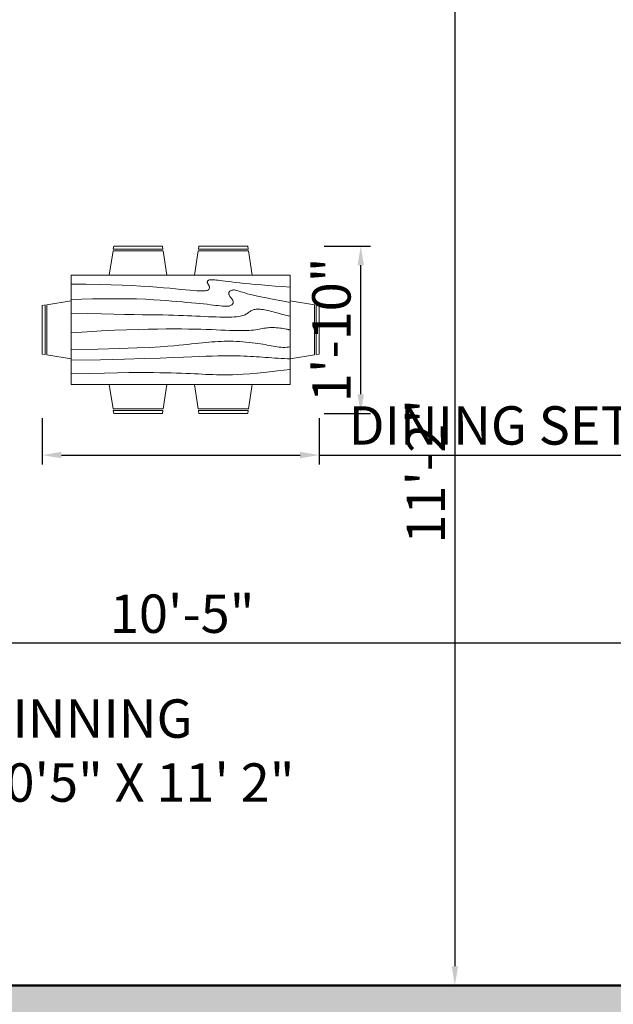
# Model space of a CAD drawing. Units: millimetres. Extents: x 2784 to 3697, y 603 to 1406.
# Tile 5 of 10: x 3013 to 3091, y 1077 to 1205. Entities that reach past the tile are written whole.
import ezdxf

# ---------------------------------------------------------------- set-up
doc = ezdxf.new("R2010")
doc.units = ezdxf.units.MM
for name, color, linetype, lineweight in [('A-ANNO-DIMS', 140, 'Continuous', 18), ('A-AREA-IDEN', 150, 'Continuous', 25), ('A-FURN', 80, 'Continuous', 18), ('A-WALL', 2, 'Continuous', 50), ('A-WALL-PATT', 8, 'Continuous', 13)]:
    doc.layers.add(name, color=color, linetype=linetype, lineweight=lineweight)
doc.styles.get("Standard").update_dxf_attribs({"font": 'arial.ttf'})
doc.dimstyles.new('ISO-25', dxfattribs={"dimtxt": 5, "dimasz": 2.5, "dimexe": 1.25, "dimexo": 0.625, "dimtad": 1, "dimdec": 0, "dimlunit": 3, "dimtxsty": 'Standard', "dimcen": 2.5, "dimadec": 0, "dimazin": 0, "dimtfac": 1, "dimtdec": 0, "dimtmove": 0, "dimatfit": 3, "dimfxl": 1, "dimarcsym": 0})

# ---------------------------------------------------------------- blocks, each defined once
blk = doc.blocks.new('Dining Set - 36 x 72 in.')
for p, q in [((-22.2343, 26.00059), (-23.4847, 17.99762)), ((-22.2304, 26), (-5.7608, 26)), ((-22, 27.5), (-22.1562, 26.50042)), ((-5.8416, 26.5), (-22.1534, 26.5)), ((-22, 27.5), (-6, 27.5)), ((-5.8437, 26.49966), (-6, 27.5)), ((-4.5152, 17.99762), (-5.7655, 25.99926)), ((5.7657, 26.00059), (4.5153, 17.99762)), ((5.7696, 26), (22.2392, 26)), ((6, 27.5), (5.8438, 26.50042)), ((22.1584, 26.5), (5.8466, 26.5)), ((6, 27.5), (22, 27.5)), ((22.1563, 26.49966), (22, 27.5)), ((23.4848, 17.99762), (22.2345, 25.99926)), ((36, 18), (-36, 18)), ((-36, 18), (-36, -18)), ((36, -18), (36, 18)), ((-45.5, 8), (-44.5004, 8.15617)), ((-45.5, 8), (-45.5, -8)), ((-44.5, -8.15843), (-44.5, 8.15338)), ((-44.0006, 8.23428), (-35.9976, 9.48474)), ((-44, 8.23041), (-44, -8.23915)), ((44.0006, 8.23428), (35.9976, 9.48474)), ((44, 8.23041), (44, -8.23915)), ((44.5, -8.15843), (44.5, 8.15338)), ((45.5, 8), (44.5005, 8.15617)), ((45.5, 8), (45.5, -8)), ((-44.4997, -8.15631), (-45.5, -8)), ((-35.9976, -9.48476), (-43.9993, -8.2345)), ((35.9976, -9.48476), (43.9993, -8.2345)), ((44.4997, -8.15631), (45.5, -8)), ((-36, -18), (36, -18)), ((-22.2343, -26.0006), (-23.4847, -17.99762)), ((-4.5152, -17.99762), (-5.7655, -25.99928)), ((5.7657, -26.0006), (4.5153, -17.99762)), ((23.4848, -17.99762), (22.2345, -25.99928)), ((-22.2304, -26), (-5.7608, -26)), ((-22, -27.5), (-22.1562, -26.50044)), ((-5.8416, -26.5), (-22.1534, -26.5)), ((-22, -27.5), (-6, -27.5)), ((-5.8437, -26.49967), (-6, -27.5)), ((5.7696, -26), (22.2392, -26)), ((6, -27.5), (5.8438, -26.50044)), ((22.1584, -26.5), (5.8466, -26.5)), ((6, -27.5), (22, -27.5)), ((22.1563, -26.49967), (22, -27.5))]:
    blk.add_line(p, q)
for points in [[(-36, 15), (-31.1772, 14.97754), (-26.8079, 14.91406), (-22.8538, 14.81543), (-19.276, 14.6875), (-16.0362, 14.53613), (-13.0957, 14.36718), (-10.4159, 14.18652), (-7.9583, 14), (-5.6904, 13.81315), (-3.6035, 13.63021), (-1.6954, 13.45508), (0.0365, 13.29166), (1.5945, 13.14388), (2.9811, 13.01562), (4.1988, 12.9108), (5.25, 12.83333), (6.1393, 12.78613), (6.8802, 12.76823), (7.4883, 12.77767), (7.9792, 12.8125), (8.3685, 12.87077), (8.6719, 12.95052), (8.9049, 13.0498), (9.0833, 13.16666), (9.2205, 13.29899), (9.3216, 13.44401), (9.3895, 13.59879), (9.4271, 13.76041), (9.4373, 13.92594), (9.4232, 14.09245), (9.3875, 14.257), (9.3333, 14.41666), (9.2638, 14.56917), (9.1836, 14.71484), (9.0975, 14.85465), (9.0104, 14.98958), (8.9272, 15.1206), (8.8529, 15.2487), (8.7922, 15.37483), (8.75, 15.5), (8.7305, 15.62467), (8.7344, 15.74739), (8.7617, 15.86621), (8.8125, 15.97916), (8.8867, 16.08431), (8.9844, 16.17968), (9.1055, 16.26334), (9.25, 16.33333), (9.4189, 16.38802), (9.6172, 16.42708), (9.8506, 16.45052), (10.125, 16.45833), (10.4463, 16.45052), (10.8203, 16.42708), (11.2529, 16.38802), (11.75, 16.33333), (12.3184, 16.26318), (12.9694, 16.17838), (13.7151, 16.07991), (14.5677, 15.96875), (15.5395, 15.84586), (16.6426, 15.71224), (17.8893, 15.56884), (19.2917, 15.41666), (20.859, 15.25667), (22.5879, 15.08984), (24.4721, 14.91715), (26.5052, 14.73958), (28.6809, 14.5581), (30.9929, 14.3737), (33.4347, 14.18733), (36, 14)], [(-36, 10), (-28.9766, 10.14274), (-23.1725, 10.20442), (-18.4241, 10.19775), (-14.5677, 10.13541), (-11.4399, 10.03011), (-8.877, 9.89453), (-6.7154, 9.74137), (-4.7917, 9.58333), (-2.9698, 9.43082), (-1.2246, 9.28515), (0.4415, 9.14534), (2.026, 9.01041), (3.5266, 8.87939), (4.9408, 8.7513), (6.266, 8.62516), (7.5, 8.5), (8.6411, 8.37549), (9.6914, 8.2539), (10.6538, 8.13818), (11.5312, 8.03125), (12.3267, 7.93603), (13.043, 7.85547), (13.6831, 7.79248), (14.25, 7.75), (14.7471, 7.7303), (15.1797, 7.73307), (15.5537, 7.75732), (15.875, 7.80208), (16.1494, 7.86637), (16.3828, 7.94922), (16.5811, 8.04964), (16.75, 8.16666), (16.8944, 8.29915), (17.0143, 8.44531), (17.1089, 8.60319), (17.1771, 8.77083), (17.218, 8.94629), (17.2305, 9.1276), (17.2137, 9.31282), (17.1667, 9.5), (17.0895, 9.6875), (16.987, 9.875), (16.8649, 10.0625), (16.7292, 10.25), (16.5856, 10.4375), (16.4401, 10.625), (16.2985, 10.8125), (16.1667, 11), (16.05, 11.18733), (15.9518, 11.3737), (15.8752, 11.5581), (15.8229, 11.73958), (15.798, 11.91715), (15.8034, 12.08984), (15.842, 12.25667), (15.9167, 12.41666), (16.0295, 12.56836), (16.1784, 12.70833), (16.3605, 12.83268), (16.5729, 12.9375), (16.8127, 13.01888), (17.0768, 13.07291), (17.3625, 13.0957), (17.6667, 13.08333), (17.9894, 13.03312), (18.3418, 12.94726), (18.7382, 12.82918), (19.1927, 12.68229), (19.7195, 12.51001), (20.3327, 12.31575), (21.0465, 12.10294), (21.875, 11.875), (22.8357, 11.63354), (23.959, 11.37304), (25.2786, 11.08618), (26.8282, 10.76562), (28.6414, 10.40405), (30.752, 9.99414), (33.1936, 9.52856), (36, 9)], [(-36, 5.5), (-30.7157, 5.3348), (-26.069, 5.20963), (-21.9946, 5.11767), (-18.4271, 5.05208), (-15.3009, 5.00602), (-12.5508, 4.97265), (-10.1112, 4.94515), (-7.9167, 4.91666), (-5.909, 4.88167), (-4.0586, 4.83984), (-2.3429, 4.79215), (-0.7396, 4.73958), (0.7739, 4.6831), (2.22, 4.6237), (3.6213, 4.56233), (5, 4.5), (6.373, 4.43782), (7.7344, 4.3776), (9.0723, 4.32129), (10.375, 4.27083), (11.6309, 4.22819), (12.8281, 4.19531), (13.9551, 4.17415), (15, 4.16666), (15.954, 4.17448), (16.819, 4.19791), (17.6001, 4.23698), (18.3021, 4.29166), (18.9299, 4.36198), (19.4883, 4.44791), (19.9823, 4.54948), (20.4167, 4.66666), (20.7969, 4.79899), (21.1302, 4.94401), (21.4245, 5.09879), (21.6875, 5.26041), (21.9271, 5.42594), (22.1511, 5.59245), (22.3672, 5.757), (22.5834, 5.91666), (22.8065, 6.06868), (23.0404, 6.21093), (23.2879, 6.34147), (23.5521, 6.45833), (23.8358, 6.55957), (24.142, 6.64323), (24.4735, 6.70735), (24.8334, 6.75), (25.2235, 6.76969), (25.642, 6.76692), (26.0858, 6.74267), (26.5521, 6.69791), (27.0379, 6.63362), (27.5404, 6.55078), (28.0565, 6.45036), (28.5834, 6.33333), (29.1242, 6.19987), (29.7071, 6.04687), (30.3661, 5.87044), (31.1354, 5.66666), (32.0493, 5.43164), (33.142, 5.16146), (34.4475, 4.85221), (36, 4.5)], [(-36, -1), (-30.7915, -0.6591), (-26.0195, -0.38216), (-21.6519, -0.16284), (-17.6563, 0.00521), (-14.0005, 0.12833), (-10.6523, 0.21289), (-7.5796, 0.26522), (-4.75, 0.29166), (-2.134, 0.29793), (0.2878, 0.28711), (2.5317, 0.26163), (4.6146, 0.22396), (6.5529, 0.17651), (8.3633, 0.12174), (10.0623, 0.06209), (11.6667, 0), (13.1899, -0.06201), (14.6341, -0.1211), (15.9982, -0.17432), (17.2813, -0.21875), (18.4823, -0.25147), (19.6003, -0.26953), (20.6343, -0.27002), (21.5834, -0.25), (22.4481, -0.20768), (23.2357, -0.14584), (23.9549, -0.06836), (24.6146, 0.02083), (25.2235, 0.11784), (25.7904, 0.21875), (26.3241, 0.31966), (26.8334, 0.41666), (27.3265, 0.50618), (27.8099, 0.58593), (28.2894, 0.65397), (28.7709, 0.70833), (29.2601, 0.74707), (29.763, 0.76823), (30.2855, 0.76985), (30.8334, 0.75), (31.4088, 0.70784), (31.9994, 0.64713), (32.589, 0.57275), (33.1615, 0.48958), (33.7008, 0.4025), (34.1908, 0.3164), (34.6153, 0.23616), (34.9584, 0.16666), (35.2099, 0.11165), (35.3848, 0.07031), (35.504, 0.04069), (35.5886, 0.02083), (35.6594, 0.00879), (35.7377, 0.0026), (35.8442, 0.00032), (36, 0)], [(-36, -6.5), (-27.1843, -6.31267), (-20.084, -6.1263), (-14.469, -5.9419), (-10.1094, -5.76042), (-6.7752, -5.58285), (-4.2363, -5.41016), (-2.2629, -5.24333), (-0.625, -5.08334), (0.8708, -4.93099), (2.2715, -4.78646), (3.5872, -4.64974), (4.8281, -4.52084), (6.0046, -4.39974), (7.127, -4.28646), (8.2053, -4.18099), (9.25, -4.08334), (10.2705, -3.99382), (11.2734, -3.91407), (12.2647, -3.84603), (13.25, -3.79167), (14.2354, -3.75293), (15.2266, -3.73177), (16.2295, -3.73015), (17.25, -3.75), (18.2912, -3.79248), (19.3451, -3.85547), (20.4009, -3.93604), (21.4479, -4.03125), (22.4754, -4.13819), (23.4727, -4.25391), (24.4289, -4.37549), (25.3334, -4.5), (26.1785, -4.62492), (26.9694, -4.74935), (27.7145, -4.87281), (28.4219, -4.99479), (29.1, -5.11483), (29.7572, -5.23242), (30.4016, -5.34709), (31.0417, -5.45834), (31.6837, -5.56437), (32.3262, -5.65821), (32.9658, -5.73153), (33.599, -5.77604), (34.2224, -5.78345), (34.8327, -5.74545), (35.4264, -5.65373), (36, -5.5)], [(-36, -10), (-26.4022, -9.81299), (-18.4675, -9.62891), (-11.9839, -9.45069), (-6.7396, -9.28125), (-2.5226, -9.12354), (0.8789, -8.98047), (3.6769, -8.85498), (6.0833, -8.75), (8.2767, -8.66765), (10.3021, -8.60677), (12.1712, -8.56543), (13.8958, -8.54167), (15.4876, -8.53353), (16.9583, -8.53907), (18.3197, -8.55632), (19.5834, -8.58334), (20.7616, -8.61841), (21.8685, -8.66081), (22.9188, -8.71004), (23.9271, -8.76563), (24.9081, -8.82707), (25.8763, -8.89388), (26.8465, -8.96558), (27.8334, -9.04167), (28.8474, -9.12118), (29.8828, -9.20117), (30.93, -9.27824), (31.9792, -9.34896), (33.0205, -9.40991), (34.0443, -9.45768), (35.0407, -9.48885), (36, -9.5)], [(-36, -14.5), (-30.0881, -14.33513), (-25.0332, -14.21224), (-20.7312, -14.12647), (-17.0781, -14.07292), (-13.97, -14.04671), (-11.3027, -14.04297), (-8.9724, -14.05681), (-6.875, -14.08334), (-4.9224, -14.11833), (-3.0905, -14.16016), (-1.3709, -14.20785), (0.2448, -14.26042), (1.7647, -14.3169), (3.1973, -14.3763), (4.5507, -14.43767), (5.8333, -14.5), (7.0554, -14.5621), (8.235, -14.62175), (9.3922, -14.67652), (10.5469, -14.72396), (11.7192, -14.76164), (12.929, -14.78711), (14.1965, -14.79794), (15.5417, -14.79167), (16.9933, -14.76424), (18.6152, -14.70508), (20.4804, -14.60197), (22.6615, -14.44271), (25.2312, -14.21509), (28.2624, -13.9069), (31.8277, -13.50594), (36, -13)]]:
    blk.add_lwpolyline(points)
blk = doc.blocks.new('*D36')
at = {"layer": 'A-ANNO-DIMS', "color": 0, "lineweight": -2, "transparency": 16777216}
for p, q in [((2971.91, 1166.33), (2971.91, 1122.59)), ((3096.91, 1166.33), (3096.91, 1122.59)), ((3094.41, 1123.84), (2974.41, 1123.84))]:
    blk.add_line(p, q, dxfattribs=at)
at = {"layer": 'A-ANNO-DIMS', "color": 0, "transparency": 16777216}
for points in [[(2974.41, 1124.26), (2974.41, 1123.43), (2971.91, 1123.84)], [(3094.41, 1124.26), (3094.41, 1123.43), (3096.91, 1123.84)]]:
    blk.add_solid(points, dxfattribs=at)
at = {"layer": 'Defpoints', "color": 0, "transparency": 16777216}
for p in [(2971.91, 1166.96), (3096.91, 1166.96), (2971.91, 1123.84)]:
    blk.add_point(p, dxfattribs=at)
at = {"layer": 'A-ANNO-DIMS', "color": 0, "transparency": 16777216, "insert": (3034.41, 1127.02), "char_height": 5, "attachment_point": 5}
blk.add_mtext('10\'-5"', dxfattribs=at)
blk = doc.blocks.new('*D37')
at = {"layer": 'A-ANNO-DIMS', "color": 0, "lineweight": -2, "transparency": 16777216}
for p, q in [((3069.6, 1213.23), (3068.7, 1213.23)), ((3069.95, 1210.73), (3069.95, 1081.73)), ((3069.6, 1079.23), (3068.7, 1079.23))]:
    blk.add_line(p, q, dxfattribs=at)
at = {"layer": 'A-ANNO-DIMS', "color": 0, "transparency": 16777216}
for points in [[(3069.53, 1210.73), (3070.37, 1210.73), (3069.95, 1213.23)], [(3069.53, 1081.73), (3070.37, 1081.73), (3069.95, 1079.23)]]:
    blk.add_solid(points, dxfattribs=at)
at = {"layer": 'Defpoints', "color": 0, "transparency": 16777216}
for p in [(3070.22, 1213.23), (3069.95, 1079.23), (3070.22, 1079.23)]:
    blk.add_point(p, dxfattribs=at)
at = {"layer": 'A-ANNO-DIMS', "color": 0, "transparency": 16777216, "insert": (3066.81, 1146.23), "char_height": 5, "attachment_point": 5, "rotation": 90}
blk.add_mtext('11\'-2"', dxfattribs=at)
blk = doc.blocks.new('*D74')
at = {"layer": 'A-ANNO-DIMS', "color": 0, "lineweight": -2, "transparency": 16777216}
for p, q in [((3016.17, 1153.13), (3016.17, 1147.09)), ((3052.27, 1153.13), (3052.27, 1147.09)), ((3018.67, 1148.34), (3049.77, 1148.34)), ((3052.27, 1148.34), (3110.98, 1148.34))]:
    blk.add_line(p, q, dxfattribs=at)
at = {"layer": 'A-ANNO-DIMS', "color": 0, "transparency": 16777216}
for points in [[(3018.67, 1148.76), (3018.67, 1147.92), (3016.17, 1148.34)], [(3049.77, 1148.76), (3049.77, 1147.92), (3052.27, 1148.34)]]:
    blk.add_solid(points, dxfattribs=at)
at = {"layer": 'Defpoints', "color": 0, "transparency": 16777216}
for p in [(3016.17, 1153.76), (3052.27, 1153.76), (3052.27, 1148.34)]:
    blk.add_point(p, dxfattribs=at)
at = {"layer": 'A-ANNO-DIMS', "color": 0, "transparency": 16777216, "insert": (3082.87, 1151.55), "char_height": 5, "attachment_point": 5}
blk.add_mtext('DINING SET 3\'-0"', dxfattribs=at)
blk = doc.blocks.new('*D75')
at = {"layer": 'A-ANNO-DIMS', "color": 0, "lineweight": -2, "transparency": 16777216}
for p, q in [((3052.9, 1175.57), (3058.94, 1175.57)), ((3057.69, 1156.26), (3057.69, 1173.07)), ((3052.9, 1153.76), (3058.94, 1153.76))]:
    blk.add_line(p, q, dxfattribs=at)
at = {"layer": 'A-ANNO-DIMS', "color": 0, "transparency": 16777216}
for points in [[(3057.27, 1173.07), (3058.1, 1173.07), (3057.69, 1175.57)], [(3057.27, 1156.26), (3058.1, 1156.26), (3057.69, 1153.76)]]:
    blk.add_solid(points, dxfattribs=at)
at = {"layer": 'Defpoints', "color": 0, "transparency": 16777216}
for p in [(3052.27, 1175.57), (3057.69, 1175.57), (3052.27, 1153.76)]:
    blk.add_point(p, dxfattribs=at)
at = {"layer": 'A-ANNO-DIMS', "color": 0, "transparency": 16777216, "insert": (3054.51, 1164.66), "char_height": 5, "attachment_point": 5, "rotation": 90}
blk.add_mtext('1\'-10"', dxfattribs=at)

msp = doc.modelspace()

# ---------------------------------------------------------------- hatches: boundary and pattern name
at = {"layer": 'A-WALL-PATT'}
h = msp.add_hatch(color=256, dxfattribs=at)
h.dxf.hatch_style = 1
h.paths.add_polyline_path([(2869.53, 1356.23), (2839.91, 1356.23), (2839.91, 1347.23), (2869.53, 1347.23)])
h.paths.add_polyline_path([(2839.91, 1356.23), (2830.91, 1356.23), (2830.91, 1347.23), (2839.91, 1347.23)])
h.paths.add_polyline_path([(2839.91, 1347.23), (2830.91, 1347.23), (2830.91, 1314.23), (2839.91, 1314.23)])
h.paths.add_polyline_path([(2839.91, 1268.19), (2830.91, 1268.19), (2830.91, 1222.23), (2839.91, 1222.23)])
h.paths.add_polyline_path([(2839.91, 1222.23), (2830.91, 1222.23), (2830.91, 1213.23), (2839.91, 1213.23)])
h.paths.add_polyline_path([(2962.91, 1222.23), (2839.91, 1222.23), (2839.91, 1213.23), (2962.91, 1213.23)])
h.paths.add_polyline_path([(2971.91, 1222.23), (2962.91, 1222.23), (2962.91, 1213.23), (2971.91, 1213.23)])
h.paths.add_polyline_path([(2971.91, 1263.23), (2962.91, 1263.23), (2962.91, 1254.23), (2971.91, 1254.23)])
h.paths.add_polyline_path([(2971.91, 1347.23), (2962.91, 1347.23), (2962.91, 1263.23), (2971.91, 1263.23)])
h.paths.add_polyline_path([(2971.91, 1356.23), (2962.91, 1356.23), (2962.91, 1347.23), (2971.91, 1347.23)])
h.paths.add_polyline_path([(2962.91, 1356.23), (2913.7, 1356.23), (2913.7, 1347.23), (2962.91, 1347.23)])
h.paths.add_polyline_path([(2982.62, 1356.23), (2971.91, 1356.23), (2971.91, 1347.23), (2982.62, 1347.23)])
h.paths.add_polyline_path([(3019.91, 1356.23), (3004.44, 1356.23), (3004.44, 1347.23), (3019.91, 1347.23)])
h.paths.add_polyline_path([(3028.91, 1356.23), (3019.91, 1356.23), (3019.91, 1347.23), (3028.91, 1347.23)])
h.paths.add_polyline_path([(3028.91, 1347.23), (3019.91, 1347.23), (3019.91, 1287.35, -0.06506), (3026.12, 1288.16), (3028.91, 1288.16)])
h.paths.add_polyline_path([(3019.91, 1263.23), (2971.91, 1263.23), (2971.91, 1254.23), (3019.91, 1254.23)])
h.paths.add_polyline_path([(3028.91, 1263.23), (3019.91, 1263.23), (3019.91, 1254.23), (3028.91, 1254.23)])
h.paths.add_polyline_path([(3028.91, 1254.23), (3019.91, 1254.23), (3019.91, 1222.23), (3028.91, 1222.23)])
h.paths.add_polyline_path([(3028.91, 1222.23), (3019.91, 1222.23), (3019.91, 1213.23), (3028.91, 1213.23)])
h.paths.add_polyline_path([(3165.91, 1222.23), (3060.65, 1222.23, -0.056956), (3061.45, 1215.23), (3061.45, 1213.23), (3165.91, 1213.23)])
h.paths.add_polyline_path([(3080.34, 1356.23), (3028.91, 1356.23), (3028.91, 1347.23), (3080.34, 1347.23)])
h.paths.add_polyline_path([(3174.91, 1347.23), (3165.91, 1347.23), (3165.91, 1311.28), (3174.91, 1311.28)])
h.paths.add_polyline_path([(3174.91, 1356.23), (3165.91, 1356.23), (3165.91, 1347.23), (3174.91, 1347.23)])
h.paths.add_polyline_path([(3165.91, 1356.23), (3123.1, 1356.23), (3123.1, 1347.23), (3165.91, 1347.23)])
h.paths.add_polyline_path([(3174.91, 1266.65), (3165.91, 1266.65), (3165.91, 1222.23), (3174.91, 1222.23)])
h.paths.add_polyline_path([(3174.91, 1222.23), (3165.91, 1222.23), (3165.91, 1213.23), (3174.91, 1213.23)])
h.paths.add_polyline_path([(3174.91, 1213.23), (3165.91, 1213.23), (3165.91, 1194.83), (3174.91, 1194.83)])
h.paths.add_polyline_path([(3105.91, 1182.92, -0.096276), (3096.91, 1180.92), (3096.91, 1148.23), (3105.91, 1148.23)])
h.paths.add_polyline_path([(3105.91, 1213.23), (3096.91, 1213.23), (3096.91, 1205.07), (3105.91, 1205.07)])
h.paths.add_polyline_path([(2971.91, 1213.23), (2962.91, 1213.23), (2962.91, 1161.09), (2971.91, 1161.09)])
h.paths.add_polyline_path([(2839.91, 1213.23), (2830.91, 1213.23), (2830.91, 1157.46), (2839.91, 1157.46)])
h.paths.add_polyline_path([(2839.91, 1108.88), (2830.91, 1108.88), (2830.91, 1042.23), (2839.91, 1042.23)])
h.paths.add_polyline_path([(2839.91, 1042.23), (2830.91, 1042.23), (2830.91, 1033.23), (2839.91, 1033.23)])
h.paths.add_polyline_path([(2881.91, 1042.23), (2839.91, 1042.23), (2839.91, 1033.23), (2881.91, 1033.23)])
h.paths.add_polyline_path([(2996.91, 1042.23), (2890.91, 1042.23), (2890.91, 1033.23), (2996.91, 1033.23)])
h.paths.add_polyline_path([(2890.91, 1042.23), (2881.91, 1042.23), (2881.91, 1033.23), (2890.91, 1033.23)])
h.paths.add_polyline_path([(2890.91, 1033.23), (2881.91, 1033.23), (2881.91, 984.23), (2890.91, 984.23)])
h.paths.add_polyline_path([(2839.91, 1033.23), (2830.91, 1033.23), (2830.91, 984.23), (2839.91, 984.23)])
h.paths.add_polyline_path([(2839.91, 984.23), (2830.91, 984.23), (2830.91, 975.23), (2839.91, 975.23)])
h.paths.add_polyline_path([(2881.91, 984.23), (2854.14, 984.23, -0.154991), (2857.05, 975.23), (2881.91, 975.23)])
h.paths.add_polyline_path([(2890.91, 984.23), (2881.91, 984.23), (2881.91, 975.23), (2890.91, 975.23)])
h.paths.add_polyline_path([(2900.85, 984.23), (2890.91, 984.23), (2890.91, 975.23), (2900.85, 975.23), (2900.85, 975.78)])
h.paths.add_polyline_path([(2996.91, 984.23), (2923.49, 984.23, -0.089525), (2925.01, 975.78), (2925.01, 975.23), (2996.91, 975.23)])
h.paths.add_polyline_path([(3165.91, 984.23), (3005.91, 984.23), (3005.91, 975.23), (3165.91, 975.23)])
h.paths.add_polyline_path([(3005.91, 1033.23), (2996.91, 1033.23), (2996.91, 984.23), (3005.91, 984.23)])
h.paths.add_polyline_path([(3005.91, 984.23), (2996.91, 984.23), (2996.91, 975.23), (3005.91, 975.23)])
h.paths.add_polyline_path([(3005.91, 1042.23), (2996.91, 1042.23), (2996.91, 1033.23), (3005.91, 1033.23)])
h.paths.add_polyline_path([(3096.91, 1079.23), (2971.91, 1079.23), (2971.91, 1070.23), (3096.91, 1070.23)])
h.paths.add_polyline_path([(2971.91, 1079.23), (2962.91, 1079.23), (2962.91, 1070.23), (2971.91, 1070.23)])
h.paths.add_polyline_path([(2971.91, 1070.23), (2962.91, 1070.23), (2962.91, 1060.28, -0.115005), (2971.91, 1066.55)])
h.paths.add_polyline_path([(2971.91, 1105.54), (2962.91, 1105.54), (2962.91, 1079.23), (2971.91, 1079.23)])
h.paths.add_polyline_path([(3165.91, 1079.23), (3105.91, 1079.23), (3105.91, 1070.23), (3165.91, 1070.23)])
h.paths.add_polyline_path([(3105.91, 1079.23), (3096.91, 1079.23), (3096.91, 1070.23), (3105.91, 1070.23)])
h.paths.add_polyline_path([(3105.91, 1148.23), (3096.91, 1148.23), (3096.91, 1139.23), (3105.91, 1139.23)])
h.paths.add_polyline_path([(3105.91, 1139.23), (3096.91, 1139.23), (3096.91, 1104.7), (3098.08, 1104.75, -0.08216), (3105.91, 1103.81)])
h.paths.add_polyline_path([(3165.91, 1148.23), (3105.91, 1148.23), (3105.91, 1139.23), (3165.91, 1139.23)])
h.paths.add_polyline_path([(3174.91, 1148.23), (3165.91, 1148.23), (3165.91, 1139.23), (3174.91, 1139.23)])
h.paths.add_polyline_path([(3174.91, 1139.23), (3165.91, 1139.23), (3165.91, 1123.86), (3174.91, 1123.86)])
h.paths.add_polyline_path([(3174.91, 1097.37), (3165.91, 1097.37), (3165.91, 1079.23), (3174.91, 1079.23)])
h.paths.add_polyline_path([(3174.91, 1079.23), (3165.91, 1079.23), (3165.91, 1070.23), (3174.91, 1070.23)])
h.paths.add_polyline_path([(3174.91, 1070.23), (3165.91, 1070.23), (3165.91, 1048.77), (3174.91, 1048.77)])
h.paths.add_polyline_path([(3174.91, 1002.74), (3165.91, 1002.74), (3165.91, 984.23), (3174.91, 984.23)])
h.paths.add_polyline_path([(3174.91, 984.23), (3165.91, 984.23), (3165.91, 975.23), (3174.91, 975.23)])
h.paths.add_polyline_path([(3174.91, 975.23), (3165.91, 975.23), (3165.91, 725.23), (3174.91, 725.23)])
h.paths.add_polyline_path([(2839.91, 975.23), (2830.91, 975.23), (2830.91, 725.23), (2839.91, 725.23)])
h.paths.add_polyline_path([(3165.91, 725.23), (2839.91, 725.23), (2839.91, 716.23), (3165.91, 716.23)])
h.paths.add_polyline_path([(3174.91, 725.23), (3165.91, 725.23), (3165.91, 716.23), (3174.91, 716.23)])
h.paths.add_polyline_path([(2839.91, 725.23), (2830.91, 725.23), (2830.91, 716.23), (2839.91, 716.23)])

# ---------------------------------------------------------------- linework, layer by layer
at = {"layer": 'A-WALL'}
msp.add_line((2962.91, 1079.23), (3174.91, 1079.23), dxfattribs=at)

# ---------------------------------------------------------------- block references
at = {"layer": 'A-FURN', "xscale": 0.3966975197891162, "yscale": 0.3966975197891162, "zscale": 0.3966975197891162}
msp.add_blockref('Dining Set - 36 x 72 in.', (3034.22, 1164.66), dxfattribs=at)

# ---------------------------------------------------------------- texts
at = {"layer": 'A-AREA-IDEN', "insert": (3007.59, 1116.5), "char_height": 5, "attachment_point": 1}
msp.add_mtext_dynamic_manual_height_columns('DINNING \\P10\'5" X 11\' 2"', width=45.9891, gutter_width=12.5, heights=[0], dxfattribs=at)

# ---------------------------------------------------------------- dimensions: what is measured, and where the dimension line sits
at = {"layer": 'A-ANNO-DIMS'}
for base, p1, p2, override, picture, middle in [((3069.95, 1079.23), (3070.22, 1213.23), (3070.22, 1079.23), {"dimclrd": 0, "dimclre": 0, "dimclrt": 0}, '*D37', (3066.81, 1146.23)), ((3057.69, 1175.57), (3052.27, 1153.76), (3052.27, 1175.57), {"dimdec": 1, "dimrnd": 0, "dimzin": 1, "dimlunit": 4, "dimfrac": 2}, '*D75', (3054.51, 1164.66))]:
    dim = msp.add_linear_dim(base=base, p1=p1, p2=p2, angle=90, dimstyle='ISO-25', override=override, dxfattribs=at)
    dim.commit()
    dim.dimension.update_dxf_attribs({"geometry": picture, "text_midpoint": middle})
dim = msp.add_linear_dim(base=(2971.91, 1123.84), p1=(3096.91, 1166.96), p2=(2971.91, 1166.96), dimstyle='ISO-25', override={"dimclrd": 0, "dimclre": 0, "dimclrt": 0}, dxfattribs=at)
dim.commit()
dim.dimension.update_dxf_attribs({"geometry": '*D36', "text_midpoint": (3034.41, 1127.02)})
dim = msp.add_linear_dim(base=(3052.27, 1148.34), p1=(3016.17, 1153.76), p2=(3052.27, 1153.76), text='DINING SET <>', dimstyle='ISO-25', override={"dimdec": 1, "dimrnd": 0, "dimzin": 1, "dimlunit": 4, "dimfrac": 2}, dxfattribs=at)
dim.commit()
dim.dimension.update_dxf_attribs({"geometry": '*D74', "text_midpoint": (3082.87, 1151.55)})

doc.saveas('drawing.dxf')
